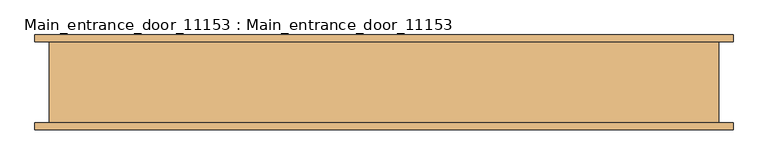
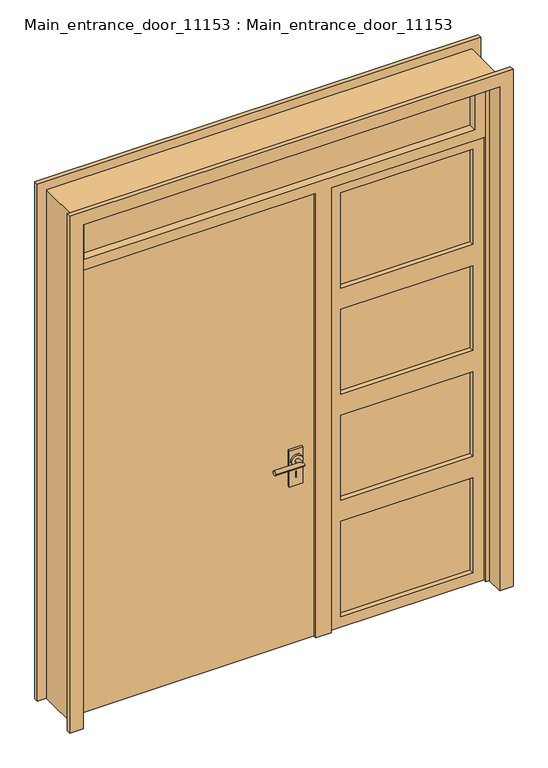
"""IFC4 building model written with IfcOpenShell, lengths in millimetres: door geometry, Main_entrance_door_11153 : Main_entrance_door_11153."""

from ifc_helpers import new_model, si_unit, point, frame, frame_2d, origin, origin_with_axes, place, context, project, spatial, polyline, circle_curve, ellipse_curve, trimmed, segment, composite_curve, outline, extrude, faceted_brep, source, transform, mapped, element, save
from ifc_brep_helpers import plane_surface, cylinder_surface, advanced_brep


def main_entrance_door_11153_main_entrance_door_11153_7490fc8c(model_context):
    return source(origin(), model_context, "Body", "SolidModel", [
        advanced_brep(
        [(60.0, -60.0, 870.0), (80.0, -60.0, 870.0), (60.0, -80.0, 870.0), (80.0, -100.0, 870.0), (-50.0, -80.0, 870.0), (-50.0, -100.0, 870.0)],
        [
            (0, 1, circle_curve(frame((70.0, -60.0, 870.0), z_axis=(0.0, 1.0, 0.0), x_axis=(1.0, 0.0, 0.0)), 10.0)),
            (1, 0, circle_curve(frame((70.0, -60.0, 870.0), z_axis=(0.0, 1.0, 0.0), x_axis=(1.0, 0.0, 0.0)), 10.0)),
            (0, 2),
            (2, 3, ellipse_curve(frame((70.0, -90.0, 870.0), z_axis=(0.7071067811865411, 0.7071067811865538, 0.0), x_axis=(-0.7071067811865538, 0.7071067811865412, 0.0)), 14.1421356, 10.0)),
            (3, 1),
            (3, 2, ellipse_curve(frame((70.0, -90.0, 870.0), z_axis=(0.7071067811865411, 0.7071067811865538, 0.0), x_axis=(-0.7071067811865538, 0.7071067811865412, 0.0)), 14.1421356, 10.0)),
            (4, 5, circle_curve(frame((-50.0, -90.0, 870.0), z_axis=(-1.0, 0.0, 0.0), x_axis=(0.0, -1.0, 0.0)), 10.0)),
            (5, 4, circle_curve(frame((-50.0, -90.0, 870.0), z_axis=(-1.0, 0.0, 0.0), x_axis=(0.0, -1.0, 0.0)), 10.0)),
            (2, 4),
            (5, 3),
        ],
        [
            plane_surface(frame((70.0, -60.0, 870.0), z_axis=(0.0, 1.0, 0.0), x_axis=(0.0, 0.0, 1.0))),
            cylinder_surface(frame((70.0, -60.0, 870.0), z_axis=(0.0, 1.0, 0.0), x_axis=(1.0, 0.0, 0.0)), 10.0),
            plane_surface(frame((-50.0, -90.0, 870.0), z_axis=(-1.0, 0.0, 0.0), x_axis=(0.0, 0.0, 1.0))),
            cylinder_surface(frame((70.0, -90.0, 870.0), z_axis=(1.0, 0.0, 0.0), x_axis=(0.0, -1.0, 0.0)), 10.0),
        ],
        [
            (0, [[1, 2]]),
            (1, [[-1, 3, 4, 5]]),
            (1, [[-2, -5, 6, -3]]),
            (2, [[7, 8]]),
            (3, [[-4, 9, -8, 10]]),
            (3, [[-6, -10, -7, -9]]),
        ],
    ),
        extrude(outline(polyline([(920.0, 100.0), (920.0, 40.0), (750.0, 40.0), (750.0, 100.0), (920.0, 100.0)]), holes=[polyline([(815.3510082, 71.5671262), (785.3510082, 71.5671262), (785.3510082, 68.4328738), (815.3510082, 68.4328738), (815.3510082, 71.5671262)])]), frame((0.0, -50.0, 0.0), z_axis=(0.0, 1.0, 0.0), x_axis=(0.0, 0.0, 1.0)), (0.0, 0.0, 1.0), 10.0),
        extrude(outline(composite_curve([segment(trimmed(circle_curve(frame_2d((870.0, 70.0)), 25.0), [point((870.0, 45.0))], [point((870.0, 95.0))], False, "CARTESIAN"), True, "CONTINUOUS"), segment(trimmed(circle_curve(frame_2d((870.0, 70.0)), 25.0), [point((870.0, 95.0))], [point((870.0, 45.0))], False, "CARTESIAN"), True, "CONTINUOUS")], self_intersect=False)), frame((0.0, -60.0, 0.0), z_axis=(0.0, 1.0, 0.0), x_axis=(0.0, 0.0, 1.0)), (0.0, 0.0, 1.0), 20.0),
        advanced_brep(
        [(60.0, 30.0, 870.0), (80.0, 30.0, 870.0), (80.0, 70.0, 870.0), (60.0, 50.0, 870.0), (-50.0, 50.0, 870.0), (-50.0, 70.0, 870.0)],
        [
            (0, 1, circle_curve(frame((70.0, 30.0, 870.0), z_axis=(0.0, -1.0, 0.0), x_axis=(1.0, 0.0, 0.0)), 10.0)),
            (1, 0, circle_curve(frame((70.0, 30.0, 870.0), z_axis=(0.0, -1.0, 0.0), x_axis=(1.0, 0.0, 0.0)), 10.0)),
            (1, 2),
            (2, 3, ellipse_curve(frame((70.0, 60.0, 870.0), z_axis=(0.7071067811865457, -0.7071067811865492, 0.0), x_axis=(-0.7071067811865492, -0.7071067811865458, 0.0)), 14.1421356, 10.0)),
            (3, 0),
            (3, 2, ellipse_curve(frame((70.0, 60.0, 870.0), z_axis=(0.7071067811865457, -0.7071067811865492, 0.0), x_axis=(-0.7071067811865492, -0.7071067811865458, 0.0)), 14.1421356, 10.0)),
            (4, 5, circle_curve(frame((-50.0, 60.0, 870.0), z_axis=(-1.0, 0.0, 0.0), x_axis=(0.0, 1.0, 0.0)), 10.0)),
            (5, 4, circle_curve(frame((-50.0, 60.0, 870.0), z_axis=(-1.0, 0.0, 0.0), x_axis=(0.0, 1.0, 0.0)), 10.0)),
            (2, 5),
            (4, 3),
        ],
        [
            plane_surface(frame((70.0, 30.0, 870.0), z_axis=(0.0, -1.0, 0.0), x_axis=(0.0, 0.0, 1.0))),
            cylinder_surface(frame((70.0, 30.0, 870.0), z_axis=(0.0, -1.0, 0.0), x_axis=(1.0, 0.0, 0.0)), 10.0),
            plane_surface(frame((-50.0, 60.0, 870.0), z_axis=(-1.0, 0.0, 0.0), x_axis=(0.0, 0.0, 1.0))),
            cylinder_surface(frame((70.0, 60.0, 870.0), z_axis=(1.0, 0.0, 0.0), x_axis=(0.0, 1.0, 0.0)), 10.0),
        ],
        [
            (0, [[1, 2]]),
            (1, [[3, 4, 5, -2]]),
            (1, [[-5, 6, -3, -1]]),
            (2, [[7, 8]]),
            (3, [[9, -7, 10, -4]]),
            (3, [[-10, -8, -9, -6]]),
        ],
    ),
        extrude(outline(polyline([(920.0, 100.0), (920.0, 40.0), (750.0, 40.0), (750.0, 100.0), (920.0, 100.0)]), holes=[polyline([(815.3510082, 71.5671262), (785.3510082, 71.5671262), (785.3510082, 68.4328738), (815.3510082, 68.4328738), (815.3510082, 71.5671262)])]), frame((0.0, 10.0, 0.0), z_axis=(0.0, 1.0, 0.0), x_axis=(0.0, 0.0, 1.0)), (0.0, 0.0, 1.0), 10.0),
        extrude(outline(composite_curve([segment(trimmed(circle_curve(frame_2d((870.0, 70.0)), 25.0), [point((870.0, 45.0))], [point((870.0, 95.0))], False, "CARTESIAN"), True, "CONTINUOUS"), segment(trimmed(circle_curve(frame_2d((870.0, 70.0)), 25.0), [point((870.0, 95.0))], [point((870.0, 45.0))], False, "CARTESIAN"), True, "CONTINUOUS")], self_intersect=False)), frame((0.0, 10.0, 0.0), z_axis=(0.0, 1.0, 0.0), x_axis=(0.0, 0.0, 1.0)), (0.0, 0.0, 1.0), 20.0),
        faceted_brep([(990.0, -114.3, 0.0), (990.0, -134.3, 0.0), (930.0, -134.3, 0.0), (930.0, -55.0, 0.0), (915.0, -55.0, 0.0), (915.0, -40.0, 0.0), (930.0, -40.0, 0.0), (930.0, 134.3, 0.0), (990.0, 134.3, 0.0), (990.0, 114.3, 0.0), (950.0, 114.3, 0.0), (950.0, -114.3, 0.0), (950.0, -114.3, 2400.0), (-950.0, -114.3, 2400.0), (-950.0, -114.3, 0.0), (-990.0, -114.3, 0.0), (-990.0, -114.3, 2440.0), (990.0, -114.3, 2440.0), (950.0, 114.3, 2400.0), (990.0, 114.3, 2440.0), (-990.0, 114.3, 2440.0), (-990.0, 114.3, 0.0), (-950.0, 114.3, 0.0), (-950.0, 114.3, 2400.0), (990.0, 134.3, 2440.0), (930.0, 134.3, 2380.0), (-930.0, 134.3, 2380.0), (-930.0, 134.3, 0.0), (-990.0, 134.3, 0.0), (-990.0, 134.3, 2440.0), (930.0, -40.0, 2380.0), (915.0, -40.0, 2365.0), (-915.0, -40.0, 2365.0), (-915.0, -40.0, 0.0), (-930.0, -40.0, 0.0), (-930.0, -40.0, 2380.0), (915.0, -55.0, 2365.0), (930.0, -55.0, 2380.0), (-930.0, -55.0, 2380.0), (-930.0, -55.0, 0.0), (-915.0, -55.0, 0.0), (-915.0, -55.0, 2365.0), (930.0, -134.3, 2380.0), (990.0, -134.3, 2440.0), (-990.0, -134.3, 2440.0), (-990.0, -134.3, 0.0), (-930.0, -134.3, 0.0), (-930.0, -134.3, 2380.0)], [[[0, 1, 2, 3, 4, 5, 6, 7, 8, 9, 10, 11]], [[11, 12, 13, 14, 15, 16, 17, 0]], [[10, 18, 12, 11]], [[9, 19, 20, 21, 22, 23, 18, 10]], [[8, 24, 19, 9]], [[7, 25, 26, 27, 28, 29, 24, 8]], [[6, 30, 25, 7]], [[5, 31, 32, 33, 34, 35, 30, 6]], [[4, 36, 31, 5]], [[3, 37, 38, 39, 40, 41, 36, 4]], [[2, 42, 37, 3]], [[1, 43, 44, 45, 46, 47, 42, 2]], [[0, 17, 43, 1]], [[15, 45, 44, 16]], [[14, 22, 21, 28, 27, 34, 33, 40, 39, 46, 45, 15]], [[13, 23, 22, 14]], [[20, 29, 28, 21]], [[26, 35, 34, 27]], [[32, 41, 40, 33]], [[38, 47, 46, 39]], [[16, 44, 43, 17]], [[12, 18, 23, 13]], [[19, 24, 29, 20]], [[25, 30, 35, 26]], [[31, 36, 41, 32]], [[37, 42, 47, 38]]]),
        faceted_brep([(225.0, -40.0, 0.0), (225.0, -55.0, 0.0), (155.0, -55.0, 0.0), (155.0, -40.0, 0.0), (170.0, -40.0, 0.0), (170.0, 10.0, 0.0), (930.0, 10.0, 0.0), (930.0, -40.0, 0.0), (930.0, -40.0, 2100.0), (225.0, -40.0, 2100.0), (865.0, -40.0, 1500.0), (865.0, -40.0, 1100.0), (275.0, -40.0, 1100.0), (275.0, -40.0, 1500.0), (865.0, -40.0, 500.0), (865.0, -40.0, 50.0), (275.0, -40.0, 50.0), (275.0, -40.0, 500.0), (865.0, -40.0, 1000.0), (865.0, -40.0, 600.0), (275.0, -40.0, 600.0), (275.0, -40.0, 1000.0), (865.0, -40.0, 2050.0), (865.0, -40.0, 1600.0), (275.0, -40.0, 1600.0), (275.0, -40.0, 2050.0), (930.0, 10.0, 2380.0), (930.0, -55.0, 2380.0), (930.0, -55.0, 2100.0), (170.0, 10.0, 2100.0), (-930.0, 10.0, 2100.0), (-930.0, 10.0, 2380.0), (275.0, 10.0, 1500.0), (275.0, 10.0, 1100.0), (865.0, 10.0, 1100.0), (865.0, 10.0, 1500.0), (275.0, 10.0, 500.0), (275.0, 10.0, 50.0), (865.0, 10.0, 50.0), (865.0, 10.0, 500.0), (275.0, 10.0, 1000.0), (275.0, 10.0, 600.0), (865.0, 10.0, 600.0), (865.0, 10.0, 1000.0), (-880.0, 10.0, 2315.0), (-880.0, 10.0, 2150.0), (865.0, 10.0, 2150.0), (865.0, 10.0, 2315.0), (275.0, 10.0, 2050.0), (275.0, 10.0, 1600.0), (865.0, 10.0, 1600.0), (865.0, 10.0, 2050.0), (170.0, -40.0, 2100.0), (155.0, -40.0, 2100.0), (155.0, -55.0, 2100.0), (225.0, -55.0, 2100.0), (-930.0, -55.0, 2380.0), (-930.0, -55.0, 2100.0), (865.0, -55.0, 2315.0), (865.0, -55.0, 2150.0), (-880.0, -55.0, 2150.0), (-880.0, -55.0, 2315.0)], [[[0, 1, 2, 3, 4, 5, 6, 7]], [[7, 8, 9, 0], [10, 11, 12, 13], [14, 15, 16, 17], [18, 19, 20, 21], [22, 23, 24, 25]], [[6, 26, 27, 28, 8, 7]], [[5, 29, 30, 31, 26, 6], [32, 33, 34, 35], [36, 37, 38, 39], [40, 41, 42, 43], [44, 45, 46, 47], [48, 49, 50, 51]], [[4, 52, 29, 5]], [[3, 53, 52, 4]], [[2, 54, 53, 3]], [[1, 55, 28, 27, 56, 57, 54, 2], [58, 59, 60, 61]], [[0, 9, 55, 1]], [[14, 17, 36, 39]], [[39, 38, 15, 14]], [[16, 15, 38, 37]], [[17, 16, 37, 36]], [[18, 21, 40, 43]], [[43, 42, 19, 18]], [[20, 19, 42, 41]], [[21, 20, 41, 40]], [[35, 34, 11, 10]], [[12, 11, 34, 33]], [[13, 12, 33, 32]], [[27, 26, 31, 56]], [[31, 30, 57, 56]], [[58, 61, 44, 47]], [[47, 46, 59, 58]], [[61, 60, 45, 44]], [[10, 13, 32, 35]], [[22, 25, 48, 51]], [[24, 23, 50, 49]], [[25, 24, 49, 48]], [[51, 50, 23, 22]], [[30, 29, 52, 53, 54, 57]], [[55, 9, 8, 28]], [[60, 59, 46, 45]]]),
        extrude(outline(polyline([(170.0, -40.0), (-930.0, -40.0), (-930.0, 10.0), (170.0, 10.0), (170.0, -40.0)])), origin_with_axes(), (0.0, 0.0, 1.0), 2100.0),
        extrude(outline(polyline([(-880.0, -12.0), (865.0, -12.0), (865.0, -18.0), (-880.0, -18.0), (-880.0, -12.0)])), frame((0.0, 0.0, 2150.0), z_axis=(0.0, 0.0, 1.0), x_axis=(1.0, 0.0, 0.0)), (0.0, 0.0, 1.0), 165.0),
        extrude(outline(polyline([(865.0, -18.0), (275.0, -18.0), (275.0, -12.0), (865.0, -12.0), (865.0, -18.0)])), frame((0.0, 0.0, 50.0), z_axis=(0.0, 0.0, 1.0), x_axis=(1.0, 0.0, 0.0)), (0.0, 0.0, 1.0), 450.0),
        extrude(outline(polyline([(865.0, -18.0), (275.0, -18.0), (275.0, -12.0), (865.0, -12.0), (865.0, -18.0)])), frame((0.0, 0.0, 600.0), z_axis=(0.0, 0.0, 1.0), x_axis=(1.0, 0.0, 0.0)), (0.0, 0.0, 1.0), 400.0),
        extrude(outline(polyline([(865.0, -18.0), (275.0, -18.0), (275.0, -12.0), (865.0, -12.0), (865.0, -18.0)])), frame((0.0, 0.0, 1600.0), z_axis=(0.0, 0.0, 1.0), x_axis=(1.0, 0.0, 0.0)), (0.0, 0.0, 1.0), 450.0),
        extrude(outline(polyline([(865.0, -18.0), (275.0, -18.0), (275.0, -12.0), (865.0, -12.0), (865.0, -18.0)])), frame((0.0, 0.0, 1100.0), z_axis=(0.0, 0.0, 1.0), x_axis=(1.0, 0.0, 0.0)), (0.0, 0.0, 1.0), 400.0),
    ])


if __name__ == "__main__":
    model = new_model("IFC4")
    model_context = context("Model", 3, world=origin())
    ifc_project = project(units=[si_unit("LENGTHUNIT", "METRE", prefix="MILLI")], contexts=[model_context])
    site = spatial("IfcSite", under=ifc_project)
    building = spatial("IfcBuilding", under=site)
    placement = place(None, origin())
    main_entrance_door_11153_main_entrance_door_11153_shape = main_entrance_door_11153_main_entrance_door_11153_7490fc8c(model_context)
    element("IfcDoor", 1, ObjectType="Main_entrance_door_11153 : Main_entrance_door_11153", at=placement, inside=building, context=model_context, shape_type="MappedRepresentation", body=[
        mapped(main_entrance_door_11153_main_entrance_door_11153_shape, transform((0.0, 0.0, 0.0), x_axis=(1.0, 0.0, 0.0), y_axis=(0.0, 1.0, 0.0), z_axis=(0.0, 0.0, 1.0))),
    ])
    save(model, "model.ifc")

# Revit data of these elements
# Type "Main_entrance_door_11153 : Main_entrance_door_11153"
#   Type Mark = "8"
#   Height = 7' - 10.48819"
#   Width = 6' - 2.80315"
#   Door Width = 3' - 7.30709"
#   Function = (empty or 0)
#   Wall Closure = (empty or 0)
# Element 1 (IfcDoor, "Main_entrance_door_11153 : Main_entrance_door_11153")
#   Materials on its faces: "Glass", "Default"
# Materials
#   "Glass": class "Glass", colour RGB 0 128 192, transparency 0.75, Description = "Soda Lime Glass", Cost = 0
#   "Default": colour RGB 127 127 127, transparency 0, Cost = 0
